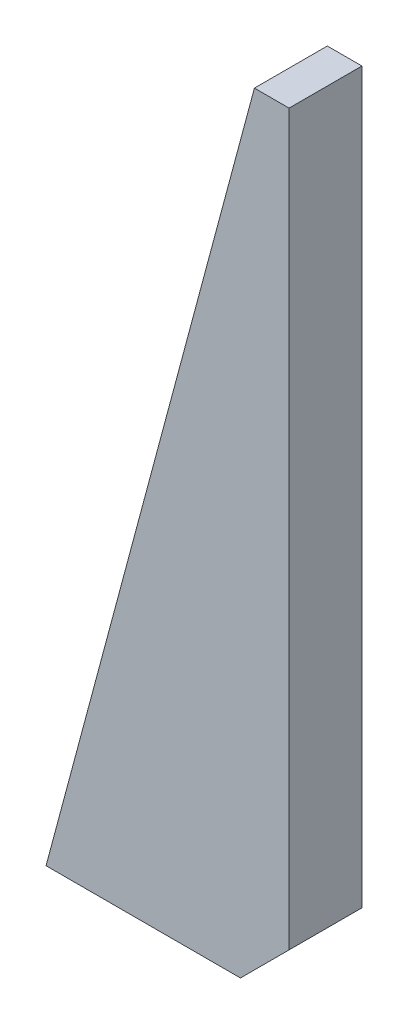
from build123d import *

# Parameters (mm, degrees)
GUSSET_PLATE_15MM_DEPTH = 15
EDGE_CHAMFER_10X45_SIZE = 10


with BuildPart() as part:
    # Gusset Profile Sketch → Gusset Plate 15mm (new body)
    with BuildSketch(Plane.XY):
        Polygon((0, 0), (-50, 0), (-7.128129211, 160), (0, 160), align=None)
    extrude(amount=GUSSET_PLATE_15MM_DEPTH)

    # Edge Chamfer 10x45
    edge_chamfer_10x45_edges = [part.edges().sort_by_distance(p)[0] for p in [
        (0, 0, 7.5),
    ]]
    chamfer(edge_chamfer_10x45_edges, length=EDGE_CHAMFER_10X45_SIZE)


solid = part.part
